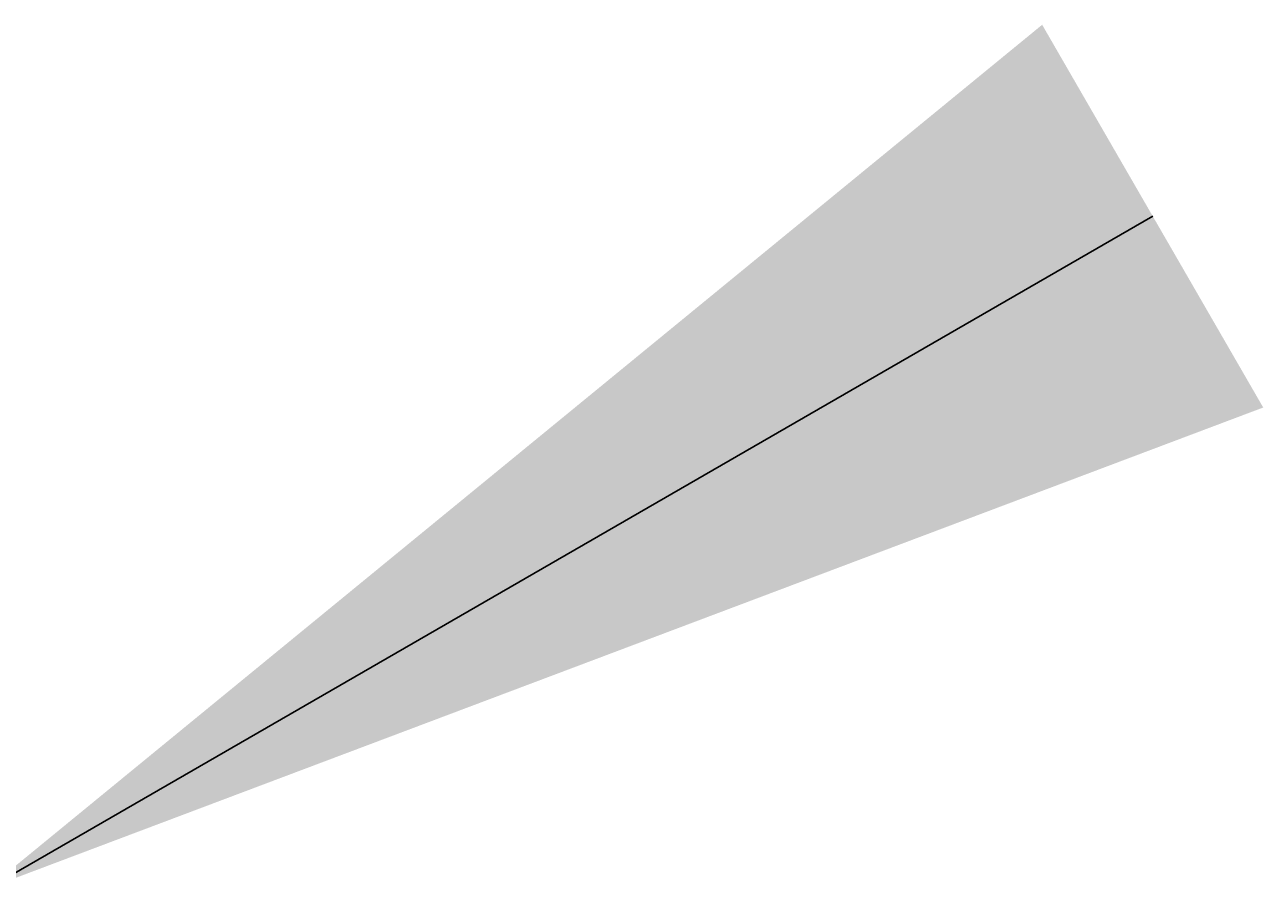
# Model space of a CAD drawing. Units: inches. Extents: x -9413 to 9703, y -9719 to 9096.
# Tile 1 of 1: x 493 to 9703, y 154 to 6578. Entities that reach past the tile are written whole.
import ezdxf
from ezdxf import colors
from ezdxf.entities.mleader import LeaderData, LeaderLine
from ezdxf.math import Vec2, Vec3

# ---------------------------------------------------------------- set-up
doc = ezdxf.new("R2010")
doc.units = ezdxf.units.IN
doc.header["$MEASUREMENT"] = 0
doc.layers.add('M-ANNO-TEXT', color=7, linetype='Continuous', lineweight=18)
doc.styles.get("Standard").update_dxf_attribs({"font": 'arial.ttf'})

msp = doc.modelspace()

# ---------------------------------------------------------------- leaders
at = {"layer": 'M-ANNO-TEXT'}
ml = msp.add_multileader_mtext('Standard', dxfattribs=at)
ml.set_content('Reheater', color=256)
ml.set_leader_properties()
ml.build(insert=Vec2(0, 0))
ml.multileader.update_dxf_attribs({"dogleg_length": 0.36, "arrow_head_size": 10000, "scale": 10})
ctx = ml.context
ctx.base_point, ctx.scale, ctx.char_height, ctx.arrow_head_size, ctx.landing_gap_size, ctx.plane_origin = Vec3(234.1414050860131, 159.7303554673012), 10, 5.4, 10000, 0.9, Vec3(221.1444910066821, 154.3050445940477)
notes = []
notes.append((ctx, [(0, (1, 1, 0), (230.5414050860131, 159.7303554673012), (1, 0), 3.599999999999999, [(0, [(221.1444910066821, 154.3050445940477)], 0, [])])]))
ctx.mtext.insert, ctx.mtext.flow_direction = Vec3(235.0414050860131, 162.4745573772603), 5
for ctx, leaders in notes:
    for number, flags, end, landing, length, lines in leaders:
        leader = LeaderData()
        leader.index, (leader.has_last_leader_line, leader.has_dogleg_vector, leader.attachment_direction) = number, flags
        leader.last_leader_point, leader.dogleg_vector, leader.dogleg_length = Vec3(end), Vec3(landing), length
        for number, points, colour, breaks in lines:
            line = LeaderLine()
            line.index, line.vertices, line.color, line.breaks = number, Vec3.list(points), colors.encode_raw_color(colour), breaks
            leader.lines.append(line)
        ctx.leaders.append(leader)

doc.saveas('drawing.dxf')
